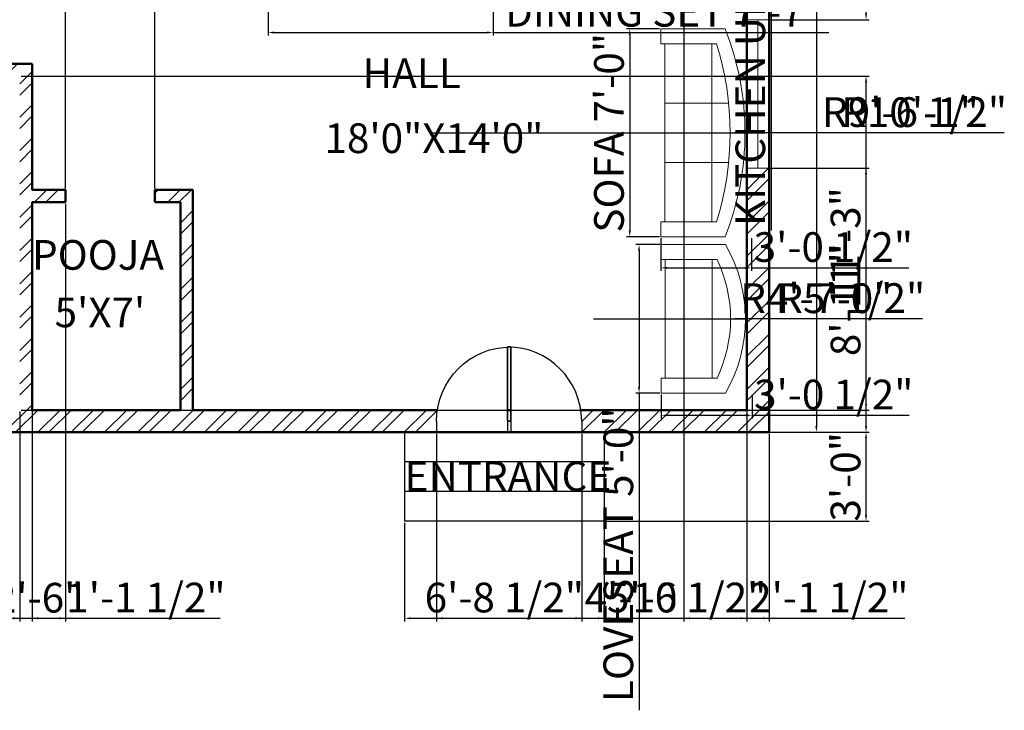
# Model space of a CAD drawing. Units: inches. Extents: x 1954 to 2815, y 1733 to 2371.
# Tile 2 of 4: x 2417 to 2815, y 1733 to 2012. Entities that reach past the tile are written whole.
import ezdxf

# ---------------------------------------------------------------- set-up
doc = ezdxf.new("R2010")
doc.units = ezdxf.units.IN
for name, color, linetype, lineweight in [('A-ANNO-DIMS', 2, 'Continuous', 18), ('A-ANNO-TEXT', 7, 'Continuous', 25), ('A-AREA-IDEN', 7, 'Continuous', 25), ('A-DOOR', 3, 'Continuous', 25), ('A-FLOR-STRS', 7, 'Continuous', 25), ('A-FURN', 8, 'Continuous', 18), ('A-GLAZ', 4, 'Continuous', 18), ('A-WALL', 7, 'Continuous', 50), ('A-WALL-PATT', 252, 'Continuous', 13)]:
    doc.layers.add(name, color=color, linetype=linetype, lineweight=lineweight)
doc.styles.get("Standard").update_dxf_attribs({"font": 'arial.ttf'})
doc.dimstyles.new('ISO-25', dxfattribs={"dimtxt": 12, "dimasz": 2.5, "dimexe": 1.25, "dimexo": 0.625, "dimtad": 1, "dimdec": 1, "dimlunit": 4, "dimtxsty": 'Standard', "dimcen": 2.5, "dimadec": 0, "dimazin": 0, "dimtfac": 1, "dimtdec": 1, "dimtmove": 0, "dimatfit": 3, "dimfxl": 1, "dimarcsym": 0})

# ---------------------------------------------------------------- blocks, each defined once
blk = doc.blocks.new('*U2')
for p, q in [((0, 0), (0, -6)), ((40, 0), (40, -6))]:
    blk.add_line(p, q)
blk.add_lwpolyline([(0, 0), (0, 40), (1.75, 40), (1.75, 0)], close=True)
blk.add_arc((0, 0), 40, 0, 90)
blk = doc.blocks.new('Sofa - Roundback Loveseat 5 ft.')
for p, q in [((0, -32.44198), (0, -5.99998)), ((-24, -33.99998), (-24, -11.46958)), ((24.00004, -33.99998), (24.00004, -11.46958)), ((-23.9998, -13.38178), (23.99986, -13.38178)), ((-24, -32.44198), (24.00004, -32.44198))]:
    blk.add_line(p, q)
for points in [[(-24, -33.99998), (-30, -33.99998), (-30, -7.99998)], [(30.00004, -7.99998), (30.00004, -33.99998), (24.00004, -33.99998)]]:
    blk.add_lwpolyline(points)
for centre, radius, start, end in [((0, -60.24998), 60.24998, 60.13715, 119.8628), ((0, -61.38438), 55.38444, 64.32083, 115.6792)]:
    blk.add_arc(centre, radius, start, end)
blk = doc.blocks.new('Sofa - Roundback 7 ft.')
for p, q in [((-12.00002, -32.4421), (-12.00003, -6.5971)), ((11.99997, -32.4421), (11.99998, -6.5971)), ((-36.000027, -34), (-36.000027, -11.4696)), ((35.99998, -34), (35.99998, -11.4696)), ((-35.999844, -13.3819), (35.9998, -13.3819)), ((-36.000027, -32.4421), (35.99998, -32.4421))]:
    blk.add_line(p, q)
for points in [[(-36.000027, -34), (-42.000027, -34), (-42.000027, -8)], [(41.99998, -8), (41.99998, -34), (35.99998, -34)]]:
    blk.add_lwpolyline(points)
for centre, radius, start, end in [((0, -114.25), 114.25, 68.43141, 111.5686), ((-0.00001, -127.1968), 121.1968, 72.72033, 107.2797)]:
    blk.add_arc(centre, radius, start, end)
blk = doc.blocks.new('*D11')
at = {"layer": 'A-ANNO-DIMS', "color": 0, "lineweight": -2, "transparency": 16777216}
for p, q in [((2720.51, 2264.98), (2740.24, 2264.98)), ((2738.99, 2262.48), (2738.99, 1847.48)), ((2720.51, 1844.98), (2740.24, 1844.98))]:
    blk.add_line(p, q, dxfattribs=at)
at = {"layer": 'A-ANNO-DIMS', "color": 0, "transparency": 16777216}
for points in [[(2738.57, 2262.48), (2739.41, 2262.48), (2738.99, 2264.98)], [(2738.57, 1847.48), (2739.41, 1847.48), (2738.99, 1844.98)]]:
    blk.add_solid(points, dxfattribs=at)
at = {"layer": 'Defpoints', "color": 0, "transparency": 16777216}
for p in [(2719.88, 2264.98), (2719.88, 1844.98), (2738.99, 1844.98)]:
    blk.add_point(p, dxfattribs=at)
at = {"layer": 'A-ANNO-DIMS', "color": 0, "transparency": 16777216, "insert": (2732.23, 2054.98), "char_height": 12, "attachment_point": 5, "rotation": 90}
blk.add_mtext("35'", dxfattribs=at)
blk = doc.blocks.new('WIN-60IN')
blk.add_line((4.5, 60), (4.5, 0))
blk.add_lwpolyline([(9, 60), (9, 0), (0, 0), (0, 60)], close=True)
blk = doc.blocks.new('*D22')
at = {"layer": 'A-ANNO-DIMS', "color": 0, "lineweight": -2, "transparency": 16777216}
for p, q in [((2710.56, 2192.43), (2721.92, 2192.43)), ((2720.67, 2189.93), (2720.67, 2123.41)), ((2710.56, 2120.91), (2721.92, 2120.91)), ((2720.67, 2120.91), (2720.67, 1926.5))]:
    blk.add_line(p, q, dxfattribs=at)
at = {"layer": 'A-ANNO-DIMS', "color": 0, "transparency": 16777216}
for points in [[(2720.25, 2189.93), (2721.08, 2189.93), (2720.67, 2192.43)], [(2720.25, 2123.41), (2721.08, 2123.41), (2720.67, 2120.91)]]:
    blk.add_solid(points, dxfattribs=at)
at = {"layer": 'Defpoints', "color": 0, "transparency": 16777216}
for p in [(2709.94, 2192.43), (2709.94, 2120.91), (2720.67, 2120.91)]:
    blk.add_point(p, dxfattribs=at)
at = {"layer": 'A-ANNO-DIMS', "color": 0, "transparency": 16777216, "insert": (2713.84, 2022.46), "char_height": 12, "attachment_point": 5, "rotation": 90}
blk.add_mtext('KITCHEN UNIT 5\'-11 1/2"', dxfattribs=at)
blk = doc.blocks.new('*D24')
at = {"layer": 'A-ANNO-DIMS', "color": 0, "lineweight": -2, "transparency": 16777216}
for p, q in [((2517.32, 2019.64), (2517.32, 2005.36)), ((2608.32, 2019.64), (2608.32, 2005.36)), ((2519.82, 2006.61), (2605.82, 2006.61)), ((2608.32, 2006.61), (2743.97, 2006.61))]:
    blk.add_line(p, q, dxfattribs=at)
at = {"layer": 'A-ANNO-DIMS', "color": 0, "transparency": 16777216}
for points in [[(2519.82, 2007.03), (2519.82, 2006.2), (2517.32, 2006.61)], [(2605.82, 2007.03), (2605.82, 2006.2), (2608.32, 2006.61)]]:
    blk.add_solid(points, dxfattribs=at)
at = {"layer": 'Defpoints', "color": 0, "transparency": 16777216}
for p in [(2517.32, 2020.26), (2608.32, 2020.26), (2608.32, 2006.61)]:
    blk.add_point(p, dxfattribs=at)
at = {"layer": 'A-ANNO-DIMS', "color": 0, "transparency": 16777216, "insert": (2677.39, 2013.44), "char_height": 12, "attachment_point": 5}
blk.add_mtext('DINING SET 7\'-7"', dxfattribs=at)
blk = doc.blocks.new('*D26')
at = {"layer": 'A-ANNO-DIMS', "color": 0, "lineweight": -2, "transparency": 16777216}
for p, q in [((2675.68, 1920.85), (2666.05, 1920.85)), ((2667.3, 1918.35), (2667.3, 1863.35)), ((2675.68, 1860.85), (2666.05, 1860.85)), ((2667.3, 1860.85), (2667.3, 1732.57))]:
    blk.add_line(p, q, dxfattribs=at)
at = {"layer": 'A-ANNO-DIMS', "color": 0, "transparency": 16777216}
for points in [[(2666.89, 1918.35), (2667.72, 1918.35), (2667.3, 1920.85)], [(2666.89, 1863.35), (2667.72, 1863.35), (2667.3, 1860.85)]]:
    blk.add_solid(points, dxfattribs=at)
at = {"layer": 'Defpoints', "color": 0, "transparency": 16777216}
for p in [(2676.3, 1920.85), (2667.3, 1860.85), (2676.3, 1860.85)]:
    blk.add_point(p, dxfattribs=at)
at = {"layer": 'A-ANNO-DIMS', "color": 0, "transparency": 16777216, "insert": (2660.47, 1795.46), "char_height": 12, "attachment_point": 5, "rotation": 90}
blk.add_mtext('LOVESEAT 5\'-0"', dxfattribs=at)
blk = doc.blocks.new('*D27')
at = {"layer": 'A-ANNO-DIMS', "color": 0, "lineweight": -2, "transparency": 16777216}
for p, q in [((2676.3, 1860.23), (2676.3, 1850.6)), ((2712.97, 1860.23), (2712.97, 1850.6)), ((2678.8, 1851.85), (2710.47, 1851.85)), ((2712.97, 1851.85), (2776.57, 1851.85))]:
    blk.add_line(p, q, dxfattribs=at)
at = {"layer": 'A-ANNO-DIMS', "color": 0, "transparency": 16777216}
for points in [[(2678.8, 1852.27), (2678.8, 1851.44), (2676.3, 1851.85)], [(2710.47, 1852.27), (2710.47, 1851.44), (2712.97, 1851.85)]]:
    blk.add_solid(points, dxfattribs=at)
at = {"layer": 'Defpoints', "color": 0, "transparency": 16777216}
for p in [(2676.3, 1860.85), (2712.97, 1860.85), (2712.97, 1851.85)]:
    blk.add_point(p, dxfattribs=at)
at = {"layer": 'A-ANNO-DIMS', "color": 0, "transparency": 16777216, "insert": (2746.02, 1858.69), "char_height": 12, "attachment_point": 5}
blk.add_mtext('3\'-0 1/2"', dxfattribs=at)
blk = doc.blocks.new('*D28')
at = {"layer": 'A-ANNO-DIMS', "color": 0, "lineweight": -2, "transparency": 16777216}
for p, q in [((2675.51, 2008.06), (2662.28, 2008.06)), ((2663.53, 2005.56), (2663.53, 1926.56)), ((2675.51, 1924.06), (2662.28, 1924.06))]:
    blk.add_line(p, q, dxfattribs=at)
at = {"layer": 'A-ANNO-DIMS', "color": 0, "transparency": 16777216}
for points in [[(2663.12, 2005.56), (2663.95, 2005.56), (2663.53, 2008.06)], [(2663.12, 1926.56), (2663.95, 1926.56), (2663.53, 1924.06)]]:
    blk.add_solid(points, dxfattribs=at)
at = {"layer": 'Defpoints', "color": 0, "transparency": 16777216}
for p in [(2676.13, 2008.06), (2663.53, 1924.06), (2676.13, 1924.06)]:
    blk.add_point(p, dxfattribs=at)
at = {"layer": 'A-ANNO-DIMS', "color": 0, "transparency": 16777216, "insert": (2656.7, 1966.06), "char_height": 12, "attachment_point": 5, "rotation": 90}
blk.add_mtext('SOFA 7\'-0"', dxfattribs=at)
blk = doc.blocks.new('*D29')
at = {"layer": 'A-ANNO-DIMS', "color": 0, "lineweight": -2, "transparency": 16777216}
for p, q in [((2676.13, 1923.44), (2676.13, 1910.21)), ((2712.8, 1923.44), (2712.8, 1910.21)), ((2678.63, 1911.46), (2710.3, 1911.46)), ((2712.8, 1911.46), (2776.4, 1911.46))]:
    blk.add_line(p, q, dxfattribs=at)
at = {"layer": 'A-ANNO-DIMS', "color": 0, "transparency": 16777216}
for points in [[(2678.63, 1911.88), (2678.63, 1911.04), (2676.13, 1911.46)], [(2710.3, 1911.88), (2710.3, 1911.04), (2712.8, 1911.46)]]:
    blk.add_solid(points, dxfattribs=at)
at = {"layer": 'Defpoints', "color": 0, "transparency": 16777216}
for p in [(2676.13, 1924.06), (2712.8, 1924.06), (2712.8, 1911.46)]:
    blk.add_point(p, dxfattribs=at)
at = {"layer": 'A-ANNO-DIMS', "color": 0, "transparency": 16777216, "insert": (2745.85, 1918.3), "char_height": 12, "attachment_point": 5}
blk.add_mtext('3\'-0 1/2"', dxfattribs=at)
blk = doc.blocks.new('*D30')
at = {"layer": 'A-ANNO-DIMS', "color": 0, "lineweight": -2, "transparency": 16777216}
for p, q in [((2248.88, 1853.36), (2248.88, 1768.53)), ((2416.88, 1853.36), (2416.88, 1768.53)), ((2251.38, 1769.78), (2414.38, 1769.78))]:
    blk.add_line(p, q, dxfattribs=at)
at = {"layer": 'A-ANNO-DIMS', "color": 0, "transparency": 16777216}
for points in [[(2251.38, 1770.2), (2251.38, 1769.37), (2248.88, 1769.78)], [(2414.38, 1770.2), (2414.38, 1769.37), (2416.88, 1769.78)]]:
    blk.add_solid(points, dxfattribs=at)
at = {"layer": 'Defpoints', "color": 0, "transparency": 16777216}
for p in [(2248.88, 1853.98), (2416.88, 1853.98), (2416.88, 1769.78)]:
    blk.add_point(p, dxfattribs=at)
at = {"layer": 'A-ANNO-DIMS', "color": 0, "transparency": 16777216, "insert": (2332.88, 1776.53), "char_height": 12, "attachment_point": 5}
blk.add_mtext('14\'-0"', dxfattribs=at)
blk = doc.blocks.new('*D31')
at = {"layer": 'A-ANNO-DIMS', "color": 0, "lineweight": -2, "transparency": 16777216}
for p, q in [((2417.51, 1988.98), (2760.33, 1988.98)), ((2759.08, 1856.48), (2759.08, 1986.48)), ((2417.51, 1853.98), (2760.33, 1853.98))]:
    blk.add_line(p, q, dxfattribs=at)
at = {"layer": 'A-ANNO-DIMS', "color": 0, "transparency": 16777216}
for points in [[(2758.67, 1986.48), (2759.5, 1986.48), (2759.08, 1988.98)], [(2758.67, 1856.48), (2759.5, 1856.48), (2759.08, 1853.98)]]:
    blk.add_solid(points, dxfattribs=at)
at = {"layer": 'Defpoints', "color": 0, "transparency": 16777216}
for p in [(2416.88, 1988.98), (2759.08, 1988.98), (2416.88, 1853.98)]:
    blk.add_point(p, dxfattribs=at)
at = {"layer": 'A-ANNO-DIMS', "color": 0, "transparency": 16777216, "insert": (2752.33, 1921.48), "char_height": 12, "attachment_point": 5, "rotation": 90}
blk.add_mtext('11\'-3"', dxfattribs=at)
blk = doc.blocks.new('*D32')
at = {"layer": 'A-ANNO-DIMS', "color": 0, "lineweight": -2, "transparency": 16777216}
for p, q in [((2572.5, 1808.36), (2572.5, 1768.53)), ((2653.15, 1808.36), (2653.15, 1768.53)), ((2575, 1769.78), (2650.65, 1769.78))]:
    blk.add_line(p, q, dxfattribs=at)
at = {"layer": 'A-ANNO-DIMS', "color": 0, "transparency": 16777216}
for points in [[(2575, 1770.2), (2575, 1769.37), (2572.5, 1769.78)], [(2650.65, 1770.2), (2650.65, 1769.37), (2653.15, 1769.78)]]:
    blk.add_solid(points, dxfattribs=at)
at = {"layer": 'Defpoints', "color": 0, "transparency": 16777216}
for p in [(2572.5, 1808.98), (2653.15, 1808.98), (2653.15, 1769.78)]:
    blk.add_point(p, dxfattribs=at)
at = {"layer": 'A-ANNO-DIMS', "color": 0, "transparency": 16777216, "insert": (2612.82, 1776.61), "char_height": 12, "attachment_point": 5}
blk.add_mtext('6\'-8 1/2"', dxfattribs=at)
blk = doc.blocks.new('*D33')
at = {"layer": 'A-ANNO-DIMS', "color": 0, "lineweight": -2, "transparency": 16777216}
for p, q in [((2653.77, 1844.98), (2760.33, 1844.98)), ((2759.08, 1811.48), (2759.08, 1842.48)), ((2653.77, 1808.98), (2760.33, 1808.98))]:
    blk.add_line(p, q, dxfattribs=at)
at = {"layer": 'A-ANNO-DIMS', "color": 0, "transparency": 16777216}
for points in [[(2758.67, 1842.48), (2759.5, 1842.48), (2759.08, 1844.98)], [(2758.67, 1811.48), (2759.5, 1811.48), (2759.08, 1808.98)]]:
    blk.add_solid(points, dxfattribs=at)
at = {"layer": 'Defpoints', "color": 0, "transparency": 16777216}
for p in [(2653.15, 1844.98), (2759.08, 1844.98), (2653.15, 1808.98)]:
    blk.add_point(p, dxfattribs=at)
at = {"layer": 'A-ANNO-DIMS', "color": 0, "transparency": 16777216, "insert": (2752.33, 1826.98), "char_height": 12, "attachment_point": 5, "rotation": 90}
blk.add_mtext('3\'-0"', dxfattribs=at)
blk = doc.blocks.new('*D34')
at = {"layer": 'A-ANNO-DIMS', "color": 0, "lineweight": -2, "transparency": 16777216}
for p, q in [((2585.41, 1844.36), (2585.41, 1768.53)), ((2644.1, 1844.36), (2644.1, 1768.53)), ((2587.91, 1769.78), (2641.6, 1769.78)), ((2644.1, 1769.78), (2717.52, 1769.78))]:
    blk.add_line(p, q, dxfattribs=at)
at = {"layer": 'A-ANNO-DIMS', "color": 0, "transparency": 16777216}
for points in [[(2587.91, 1770.2), (2587.91, 1769.37), (2585.41, 1769.78)], [(2641.6, 1770.2), (2641.6, 1769.37), (2644.1, 1769.78)]]:
    blk.add_solid(points, dxfattribs=at)
at = {"layer": 'Defpoints', "color": 0, "transparency": 16777216}
for p in [(2585.41, 1844.98), (2644.1, 1844.98), (2644.1, 1769.78)]:
    blk.add_point(p, dxfattribs=at)
at = {"layer": 'A-ANNO-DIMS', "color": 0, "transparency": 16777216, "insert": (2682.06, 1776.61), "char_height": 12, "attachment_point": 5}
blk.add_mtext('4\'-10 1/2"', dxfattribs=at)
blk = doc.blocks.new('*D35')
at = {"layer": 'A-ANNO-DIMS', "color": 0, "lineweight": -2, "transparency": 16777216}
for p, q in [((2653.15, 1844.36), (2653.15, 1768.53)), ((2719.88, 1844.36), (2719.88, 1768.53)), ((2655.65, 1769.78), (2717.38, 1769.78))]:
    blk.add_line(p, q, dxfattribs=at)
at = {"layer": 'A-ANNO-DIMS', "color": 0, "transparency": 16777216}
for points in [[(2655.65, 1770.2), (2655.65, 1769.37), (2653.15, 1769.78)], [(2717.38, 1770.2), (2717.38, 1769.37), (2719.88, 1769.78)]]:
    blk.add_solid(points, dxfattribs=at)
at = {"layer": 'Defpoints', "color": 0, "transparency": 16777216}
for p in [(2653.15, 1844.98), (2719.88, 1844.98), (2719.88, 1769.78)]:
    blk.add_point(p, dxfattribs=at)
at = {"layer": 'A-ANNO-DIMS', "color": 0, "transparency": 16777216, "insert": (2686.52, 1776.61), "char_height": 12, "attachment_point": 5}
blk.add_mtext('5\'-6 1/2"', dxfattribs=at)
blk = doc.blocks.new('*D45')
at = {"layer": 'A-ANNO-DIMS', "color": 0, "lineweight": -2, "transparency": 16777216}
for p, q in [((2720.51, 2153), (2760.33, 2153)), ((2759.08, 2014.3), (2759.08, 2150.5)), ((2720.51, 2011.8), (2760.33, 2011.8))]:
    blk.add_line(p, q, dxfattribs=at)
at = {"layer": 'A-ANNO-DIMS', "color": 0, "transparency": 16777216}
for points in [[(2758.67, 2150.5), (2759.5, 2150.5), (2759.08, 2153)], [(2758.67, 2014.3), (2759.5, 2014.3), (2759.08, 2011.8)]]:
    blk.add_solid(points, dxfattribs=at)
at = {"layer": 'Defpoints', "color": 0, "transparency": 16777216}
for p in [(2719.88, 2153), (2759.08, 2153), (2719.88, 2011.8)]:
    blk.add_point(p, dxfattribs=at)
at = {"layer": 'A-ANNO-DIMS', "color": 0, "transparency": 16777216, "insert": (2752.33, 2082.4), "char_height": 12, "attachment_point": 5, "rotation": 90}
blk.add_mtext('11\'-9"', dxfattribs=at)
blk = doc.blocks.new('*D46')
at = {"layer": 'A-ANNO-DIMS', "color": 0, "lineweight": -2, "transparency": 16777216}
for p, q in [((2720.51, 1951.8), (2760.33, 1951.8)), ((2759.08, 1847.48), (2759.08, 1949.3)), ((2720.51, 1844.98), (2760.33, 1844.98))]:
    blk.add_line(p, q, dxfattribs=at)
at = {"layer": 'A-ANNO-DIMS', "color": 0, "transparency": 16777216}
for points in [[(2758.67, 1949.3), (2759.5, 1949.3), (2759.08, 1951.8)], [(2758.67, 1847.48), (2759.5, 1847.48), (2759.08, 1844.98)]]:
    blk.add_solid(points, dxfattribs=at)
at = {"layer": 'Defpoints', "color": 0, "transparency": 16777216}
for p in [(2719.88, 1951.8), (2759.08, 1951.8), (2719.88, 1844.98)]:
    blk.add_point(p, dxfattribs=at)
at = {"layer": 'A-ANNO-DIMS', "color": 0, "transparency": 16777216, "insert": (2752.33, 1898.39), "char_height": 12, "attachment_point": 5, "rotation": 90}
blk.add_mtext('8\'-11"', dxfattribs=at)
blk = doc.blocks.new('*D47')
at = {"layer": 'A-ANNO-DIMS', "color": 0, "lineweight": -2, "transparency": 16777216}
for p, q in [((2375.36, 2106.36), (2375.36, 1768.53)), ((2405.36, 2106.36), (2405.36, 1768.53)), ((2377.86, 1769.78), (2402.86, 1769.78)), ((2405.36, 1769.78), (2441.21, 1769.78))]:
    blk.add_line(p, q, dxfattribs=at)
at = {"layer": 'A-ANNO-DIMS', "color": 0, "transparency": 16777216}
for points in [[(2377.86, 1770.2), (2377.86, 1769.37), (2375.36, 1769.78)], [(2402.86, 1770.2), (2402.86, 1769.37), (2405.36, 1769.78)]]:
    blk.add_solid(points, dxfattribs=at)
at = {"layer": 'Defpoints', "color": 0, "transparency": 16777216}
for p in [(2375.36, 2106.98), (2405.36, 2106.98), (2405.36, 1769.78)]:
    blk.add_point(p, dxfattribs=at)
at = {"layer": 'A-ANNO-DIMS', "color": 0, "transparency": 16777216, "insert": (2424.53, 1776.53), "char_height": 12, "attachment_point": 5}
blk.add_mtext('2\'-6"', dxfattribs=at)
blk = doc.blocks.new('*D51')
at = {"layer": 'A-ANNO-DIMS', "color": 0, "lineweight": -2, "transparency": 16777216}
for p, q in [((2685.45, 2111.36), (2685.45, 1768.53)), ((2710.88, 2111.36), (2710.88, 1768.53)), ((2687.95, 1769.78), (2708.38, 1769.78)), ((2710.88, 1769.78), (2774.7, 1769.78))]:
    blk.add_line(p, q, dxfattribs=at)
at = {"layer": 'A-ANNO-DIMS', "color": 0, "transparency": 16777216}
for points in [[(2687.95, 1770.2), (2687.95, 1769.37), (2685.45, 1769.78)], [(2708.38, 1770.2), (2708.38, 1769.37), (2710.88, 1769.78)]]:
    blk.add_solid(points, dxfattribs=at)
at = {"layer": 'Defpoints', "color": 0, "transparency": 16777216}
for p in [(2685.45, 2111.98), (2710.88, 2111.98), (2710.88, 1769.78)]:
    blk.add_point(p, dxfattribs=at)
at = {"layer": 'A-ANNO-DIMS', "color": 0, "transparency": 16777216, "insert": (2744.04, 1776.61), "char_height": 12, "attachment_point": 5}
blk.add_mtext('2\'-1 1/2"', dxfattribs=at)
blk = doc.blocks.new('*D53')
at = {"layer": 'A-ANNO-DIMS', "color": 0, "lineweight": -2, "transparency": 16777216}
for p, q in [((2435.43, 1943.61), (2435.43, 2305.43)), ((2471.49, 1943.61), (2471.49, 2305.43)), ((2437.93, 2304.18), (2468.99, 2304.18))]:
    blk.add_line(p, q, dxfattribs=at)
at = {"layer": 'A-ANNO-DIMS', "color": 0, "transparency": 16777216}
for points in [[(2437.93, 2304.6), (2437.93, 2303.77), (2435.43, 2304.18)], [(2468.99, 2304.6), (2468.99, 2303.77), (2471.49, 2304.18)]]:
    blk.add_solid(points, dxfattribs=at)
at = {"layer": 'Defpoints', "color": 0, "transparency": 16777216}
for p in [(2471.49, 2304.18), (2435.43, 1942.98), (2471.49, 1942.98)]:
    blk.add_point(p, dxfattribs=at)
at = {"layer": 'A-ANNO-DIMS', "color": 0, "transparency": 16777216, "insert": (2453.46, 2310.94), "char_height": 12, "attachment_point": 5}
blk.add_mtext('3\'-0"', dxfattribs=at)
blk = doc.blocks.new('*D54')
at = {"layer": 'A-ANNO-DIMS', "color": 0, "lineweight": -2, "transparency": 16777216}
for p, q in [((2421.88, 1937.36), (2421.88, 1768.53)), ((2435.43, 1937.36), (2435.43, 1768.53)), ((2424.38, 1769.78), (2432.93, 1769.78)), ((2435.43, 1769.78), (2497.92, 1769.78))]:
    blk.add_line(p, q, dxfattribs=at)
at = {"layer": 'A-ANNO-DIMS', "color": 0, "transparency": 16777216}
for points in [[(2424.38, 1770.2), (2424.38, 1769.37), (2421.88, 1769.78)], [(2432.93, 1770.2), (2432.93, 1769.37), (2435.43, 1769.78)]]:
    blk.add_solid(points, dxfattribs=at)
at = {"layer": 'Defpoints', "color": 0, "transparency": 16777216}
for p in [(2421.88, 1937.98), (2435.43, 1937.98), (2435.43, 1769.78)]:
    blk.add_point(p, dxfattribs=at)
at = {"layer": 'A-ANNO-DIMS', "color": 0, "transparency": 16777216, "insert": (2467.92, 1776.61), "char_height": 12, "attachment_point": 5}
blk.add_mtext('1\'-1 1/2"', dxfattribs=at)
blk = doc.blocks.new('*D55')
at = {"layer": 'A-ANNO-DIMS', "color": 0, "lineweight": -2, "transparency": 16777216}
for p, q in [((2343.88, 1989.61), (2343.88, 2305.43)), ((2372.59, 1990.74), (2372.59, 2305.43)), ((2346.38, 2304.18), (2370.09, 2304.18)), ((2372.59, 2304.18), (2436.4, 2304.18))]:
    blk.add_line(p, q, dxfattribs=at)
at = {"layer": 'A-ANNO-DIMS', "color": 0, "transparency": 16777216}
for points in [[(2346.38, 2304.6), (2346.38, 2303.77), (2343.88, 2304.18)], [(2370.09, 2304.6), (2370.09, 2303.77), (2372.59, 2304.18)]]:
    blk.add_solid(points, dxfattribs=at)
at = {"layer": 'Defpoints', "color": 0, "transparency": 16777216}
for p in [(2372.59, 2304.18), (2343.88, 1988.98), (2372.59, 1990.12)]:
    blk.add_point(p, dxfattribs=at)
at = {"layer": 'A-ANNO-DIMS', "color": 0, "transparency": 16777216, "insert": (2405.75, 2311.01), "char_height": 12, "attachment_point": 5}
blk.add_mtext('2\'-4 1/2"', dxfattribs=at)
blk = doc.blocks.new('*D57')
at = {"layer": 'A-ANNO-DIMS', "color": 0, "lineweight": -2, "transparency": 16777216}
for p, q in [((2582.94, 1966.06), (2704.13, 1966.06)), ((2803.83, 1966.06), (2706.63, 1966.06))]:
    blk.add_line(p, q, dxfattribs=at)
at = {"layer": 'A-ANNO-DIMS', "color": 0, "transparency": 16777216}
blk.add_solid([(2706.63, 1966.48), (2706.63, 1965.64), (2704.13, 1966.06)], dxfattribs=at)
at = {"layer": 'Defpoints', "color": 0, "transparency": 16777216}
for p in [(2582.94, 1966.06), (2704.13, 1966.06)]:
    blk.add_point(p, dxfattribs=at)
at = {"layer": 'A-ANNO-DIMS', "color": 0, "transparency": 16777216, "insert": (2776.85, 1972.81), "char_height": 12, "attachment_point": 5, "rotation": 359.9998}
blk.add_mtext('R10\'-1"', dxfattribs=at)
blk = doc.blocks.new('*D58')
at = {"layer": 'A-ANNO-DIMS', "color": 0, "lineweight": -2, "transparency": 16777216}
for p, q in [((2595.88, 1966.06), (2710.13, 1966.06)), ((2814.98, 1966.06), (2712.63, 1966.06))]:
    blk.add_line(p, q, dxfattribs=at)
at = {"layer": 'A-ANNO-DIMS', "color": 0, "transparency": 16777216}
blk.add_solid([(2712.63, 1966.48), (2712.63, 1965.64), (2710.13, 1966.06)], dxfattribs=at)
at = {"layer": 'Defpoints', "color": 0, "transparency": 16777216}
for p in [(2595.88, 1966.06), (2710.13, 1966.06)]:
    blk.add_point(p, dxfattribs=at)
at = {"layer": 'A-ANNO-DIMS', "color": 0, "transparency": 16777216, "insert": (2778.68, 1972.89), "char_height": 12, "attachment_point": 5, "rotation": 359.9998}
blk.add_mtext('R9\'-6 1/2"', dxfattribs=at)
blk = doc.blocks.new('*D59')
at = {"layer": 'A-ANNO-DIMS', "color": 0, "lineweight": -2, "transparency": 16777216}
for p, q in [((2650.05, 1890.85), (2710.3, 1890.85)), ((2768.77, 1890.85), (2712.8, 1890.85))]:
    blk.add_line(p, q, dxfattribs=at)
at = {"layer": 'A-ANNO-DIMS', "color": 0, "transparency": 16777216}
blk.add_solid([(2712.8, 1891.27), (2712.8, 1890.44), (2710.3, 1890.85)], dxfattribs=at)
at = {"layer": 'Defpoints', "color": 0, "transparency": 16777216}
for p in [(2650.05, 1890.85), (2710.3, 1890.85)]:
    blk.add_point(p, dxfattribs=at)
at = {"layer": 'A-ANNO-DIMS', "color": 0, "transparency": 16777216, "insert": (2746.45, 1897.61), "char_height": 12, "attachment_point": 5, "rotation": 0.0003}
blk.add_mtext('R5\'-0"', dxfattribs=at)
blk = doc.blocks.new('*D60')
at = {"layer": 'A-ANNO-DIMS', "color": 0, "lineweight": -2, "transparency": 16777216}
for p, q in [((2648.92, 1890.85), (2704.3, 1890.85)), ((2781.9, 1890.85), (2706.8, 1890.85))]:
    blk.add_line(p, q, dxfattribs=at)
at = {"layer": 'A-ANNO-DIMS', "color": 0, "transparency": 16777216}
blk.add_solid([(2706.8, 1891.27), (2706.8, 1890.44), (2704.3, 1890.85)], dxfattribs=at)
at = {"layer": 'Defpoints', "color": 0, "transparency": 16777216}
for p in [(2648.92, 1890.85), (2704.3, 1890.85)]:
    blk.add_point(p, dxfattribs=at)
at = {"layer": 'A-ANNO-DIMS', "color": 0, "transparency": 16777216, "insert": (2745.6, 1897.68), "char_height": 12, "attachment_point": 5, "rotation": 0.0003}
blk.add_mtext('R4\'-7 1/2"', dxfattribs=at)

msp = doc.modelspace()

# ---------------------------------------------------------------- hatches: boundary and pattern name
at = {"layer": 'A-WALL-PATT'}
h = msp.add_hatch(dxfattribs=at)
h.set_pattern_fill('ANSI32', color=256)
h.paths.add_polyline_path([(2585.41, 1844.98), (2585.41, 1849.48, -0.03766), (2585.75, 1853.98), (2486.88, 1853.98), (2486.88, 1942.98), (2471.49, 1942.98), (2471.49, 1937.98), (2481.88, 1937.98), (2481.88, 1853.98), (2421.88, 1853.98), (2421.88, 1937.98), (2435.43, 1937.98), (2435.43, 1942.98), (2421.88, 1942.98), (2421.88, 1993.98), (2402.59, 1993.98), (2402.59, 1990.12, -0.009455), (2402.57, 1988.98), (2416.88, 1988.98), (2416.88, 1853.98), (2368.9, 1853.98), (2368.9, 1844.98)])
h.paths.add_polyline_path([(2308.9, 1844.98), (2308.9, 1853.98), (2248.88, 1853.98), (2248.88, 1929.98), (2343.88, 1929.98), (2343.88, 1952.31), (2339.38, 1952.31), (2338.88, 1952.31), (2338.88, 1934.98), (2248.88, 1934.98), (2248.88, 1953.35), (2239.88, 1953.35), (2239.88, 1844.98)])
h = msp.add_hatch(dxfattribs=at)
h.set_pattern_fill('ANSI32', color=256)
h.paths.add_polyline_path([(2719.88, 1951.8), (2710.88, 1951.8), (2710.88, 1853.98), (2643.76, 1853.98, -0.03766), (2644.1, 1849.48), (2644.1, 1844.98), (2719.88, 1844.98)])

# ---------------------------------------------------------------- linework, layer by layer
at = {"layer": 'A-FLOR-STRS'}
for p, q in [((2572.5, 1844.98), (2572.5, 1808.98)), ((2653.15, 1844.98), (2653.15, 1808.98)), ((2653.15, 1832.98), (2572.5, 1832.98)), ((2653.15, 1820.98), (2572.5, 1820.98)), ((2653.15, 1808.98), (2572.5, 1808.98))]:
    msp.add_line(p, q, dxfattribs=at)
at = {"layer": 'A-WALL'}
for p, q in [((2719.88, 2264.98), (2719.88, 1844.98)), ((2710.88, 2106.98), (2710.88, 1853.98)), ((2343.88, 1993.98), (2421.88, 1993.98)), ((2421.88, 1942.98), (2421.88, 1993.98)), ((2435.43, 1942.98), (2421.88, 1942.98)), ((2435.43, 1937.98), (2435.43, 1942.98)), ((2486.88, 1942.98), (2471.49, 1942.98)), ((2471.49, 1937.98), (2471.49, 1942.98)), ((2486.88, 1853.98), (2486.88, 1942.98)), ((2421.88, 1853.98), (2421.88, 1937.98)), ((2435.43, 1937.98), (2421.88, 1937.98)), ((2481.88, 1937.98), (2471.49, 1937.98)), ((2481.88, 1853.98), (2481.88, 1937.98)), ((2481.88, 1853.98), (2421.88, 1853.98)), ((2585.75, 1853.98), (2486.88, 1853.98)), ((2615.41, 1853.98), (2614.1, 1853.98)), ((2710.88, 1853.98), (2643.76, 1853.98)), ((2719.88, 1844.98), (2239.88, 1844.98))]:
    msp.add_line(p, q, dxfattribs=at)

# ---------------------------------------------------------------- block references
at = {"layer": 'A-DOOR', "yscale": 0.75, "zscale": 0.75}
for p, xscale in [((2615.41, 1849.48), -0.75), ((2614.1, 1849.48), 0.75)]:
    msp.add_blockref('*U2', p, dxfattribs=dict(at, xscale=xscale))
at = {"layer": 'A-FURN', "rotation": 270}
for name, p in [('Sofa - Roundback 7 ft.', (2710.13, 1966.06)), ('Sofa - Roundback Loveseat 5 ft.', (2710.3, 1890.85))]:
    msp.add_blockref(name, p, dxfattribs=at)
at = {"layer": 'A-GLAZ'}
msp.add_blockref('WIN-60IN', (2710.88, 1951.8), dxfattribs=at)

# ---------------------------------------------------------------- texts
at = {"layer": 'A-ANNO-TEXT'}
msp.add_text('ENTRANCE', height=12, dxfattribs=at).set_placement((2572.5, 1821.19))
at = {"layer": 'A-AREA-IDEN'}
for s, p in [('HALL', (2555.56, 1984.15)), ('18\'0"X14\'0"', (2540.1, 1957.88)), ('POOJA', (2421.88, 1910.7)), ("5'X7'", (2431, 1887.45))]:
    msp.add_text(s, height=12, dxfattribs=at).set_placement(p)

# ---------------------------------------------------------------- dimensions: what is measured, and where the dimension line sits
at = {"layer": 'A-ANNO-DIMS'}
for base, p1, p2, picture, middle in [((2372.59, 2304.18), (2343.88, 1988.98), (2372.59, 1990.12), '*D55', (2405.75, 2311.01)), ((2471.49, 2304.18), (2435.43, 1942.98), (2471.49, 1942.98), '*D53', (2453.46, 2310.94)), ((2710.88, 1769.78), (2685.45, 2111.98), (2710.88, 2111.98), '*D51', (2744.04, 1776.61)), ((2405.36, 1769.78), (2375.36, 2106.98), (2405.36, 2106.98), '*D47', (2424.53, 1776.53)), ((2435.434, 1769.783), (2421.8844, 1937.983), (2435.434, 1937.983), '*D54', (2467.9246, 1776.6126)), ((2712.8, 1911.46), (2676.13, 1924.06), (2712.8, 1924.06), '*D29', (2745.85, 1918.3)), ((2712.97, 1851.85), (2676.3, 1860.85), (2712.97, 1860.85), '*D27', (2746.02, 1858.69)), ((2416.88, 1769.78), (2248.88, 1853.98), (2416.88, 1853.98), '*D30', (2332.88, 1776.53)), ((2644.1, 1769.78), (2585.41, 1844.98), (2644.1, 1844.98), '*D34', (2682.06, 1776.61)), ((2719.88, 1769.78), (2653.15, 1844.98), (2719.88, 1844.98), '*D35', (2686.52, 1776.61)), ((2653.1475, 1769.783), (2572.5013, 1808.983), (2653.1475, 1808.983), '*D32', (2612.8244, 1776.6126))]:
    dim = msp.add_linear_dim(base=base, p1=p1, p2=p2, dimstyle='ISO-25', override={"dimdec": 1, "dimlfac": 1, "dimrnd": 0, "dimzin": 1, "dimdsep": 46, "dimlunit": 4, "dimfrac": 2}, dxfattribs=at)
    dim.commit()
    dim.dimension.update_dxf_attribs({"geometry": picture, "text_midpoint": middle})
for base, p1, p2, override, picture, middle in [((2738.99, 1844.98), (2719.88, 2264.98), (2719.88, 1844.98), {"dimclrd": 0, "dimclre": 0, "dimclrt": 0}, '*D11', (2732.23, 2054.98)), ((2759.08, 2153), (2719.88, 2011.8), (2719.88, 2153), {"dimdec": 1, "dimlfac": 1, "dimrnd": 0, "dimzin": 1, "dimdsep": 46, "dimlunit": 4, "dimfrac": 2}, '*D45', (2752.33, 2082.4)), ((2759.08, 1988.98), (2416.88, 1853.98), (2416.88, 1988.98), {"dimdec": 1, "dimlfac": 1, "dimrnd": 0, "dimzin": 1, "dimdsep": 46, "dimlunit": 4, "dimfrac": 2}, '*D31', (2752.33, 1921.48)), ((2759.08, 1951.8), (2719.88, 1844.98), (2719.88, 1951.8), {"dimdec": 1, "dimlfac": 1, "dimrnd": 0, "dimzin": 1, "dimdsep": 46, "dimlunit": 4, "dimfrac": 2}, '*D46', (2752.33, 1898.39)), ((2759.08, 1844.98), (2653.15, 1808.98), (2653.15, 1844.98), {"dimdec": 1, "dimlfac": 1, "dimrnd": 0, "dimzin": 1, "dimdsep": 46, "dimlunit": 4, "dimfrac": 2}, '*D33', (2752.33, 1826.98))]:
    dim = msp.add_linear_dim(base=base, p1=p1, p2=p2, angle=90, dimstyle='ISO-25', override=override, dxfattribs=at)
    dim.commit()
    dim.dimension.update_dxf_attribs({"geometry": picture, "text_midpoint": middle})
for base, p1, p2, text, picture, middle in [((2720.67, 2120.91), (2709.94, 2192.43), (2709.94, 2120.91), 'KITCHEN UNIT <>', '*D22', (2713.84, 2022.46)), ((2663.53, 1924.06), (2676.13, 2008.06), (2676.13, 1924.06), 'SOFA <>', '*D28', (2656.7, 1966.06)), ((2667.3, 1860.85), (2676.3, 1920.85), (2676.3, 1860.85), 'LOVESEAT <>', '*D26', (2660.47, 1795.46))]:
    dim = msp.add_linear_dim(base=base, p1=p1, p2=p2, angle=270, text=text, dimstyle='ISO-25', override={"dimdec": 1, "dimlfac": 1, "dimrnd": 0, "dimzin": 1, "dimdsep": 46, "dimlunit": 4, "dimfrac": 2}, dxfattribs=at)
    dim.commit()
    dim.dimension.update_dxf_attribs({"geometry": picture, "text_midpoint": middle})
dim = msp.add_linear_dim(base=(2608.32, 2006.61), p1=(2517.32, 2020.26), p2=(2608.32, 2020.26), text='DINING SET <>', dimstyle='ISO-25', override={"dimdec": 1, "dimlfac": 1, "dimrnd": 0, "dimzin": 1, "dimdsep": 46, "dimlunit": 4, "dimfrac": 2}, dxfattribs=at)
dim.commit()
dim.dimension.update_dxf_attribs({"geometry": '*D24', "text_midpoint": (2677.39, 2013.44)})
for center, mpoint, picture, middle in [((2595.882429, 1966.06139), (2710.132429, 1966.061), '*D58', (2778.682429, 1966.060766)), ((2582.94, 1966.06), (2704.13, 1966.06), '*D57', (2776.85, 1966.06)), ((2650.0536, 1890.8527), (2710.30358, 1890.853), '*D59', (2746.45357, 1890.85318))]:
    dim = msp.add_radius_dim(center=center, mpoint=mpoint, dimstyle='ISO-25', override={"dimdec": 1, "dimlfac": 1, "dimrnd": 0, "dimzin": 1, "dimdsep": 46, "dimlunit": 4, "dimfrac": 2}, dxfattribs=at)
    dim.commit()
    dim.dimension.update_dxf_attribs({"geometry": picture, "text_midpoint": middle, "dimtype": 164})
dim = msp.add_radius_dim(center=(2648.92, 1890.85), mpoint=(2704.3, 1890.85), dimstyle='ISO-25', override={"dimdec": 1, "dimlfac": 1, "dimrnd": 0, "dimzin": 1, "dimdsep": 46, "dimlunit": 4, "dimfrac": 2}, dxfattribs=at)
dim.commit()
dim.dimension.update_dxf_attribs({"geometry": '*D60', "text_midpoint": (2745.6, 1897.68)})

doc.saveas('drawing.dxf')
